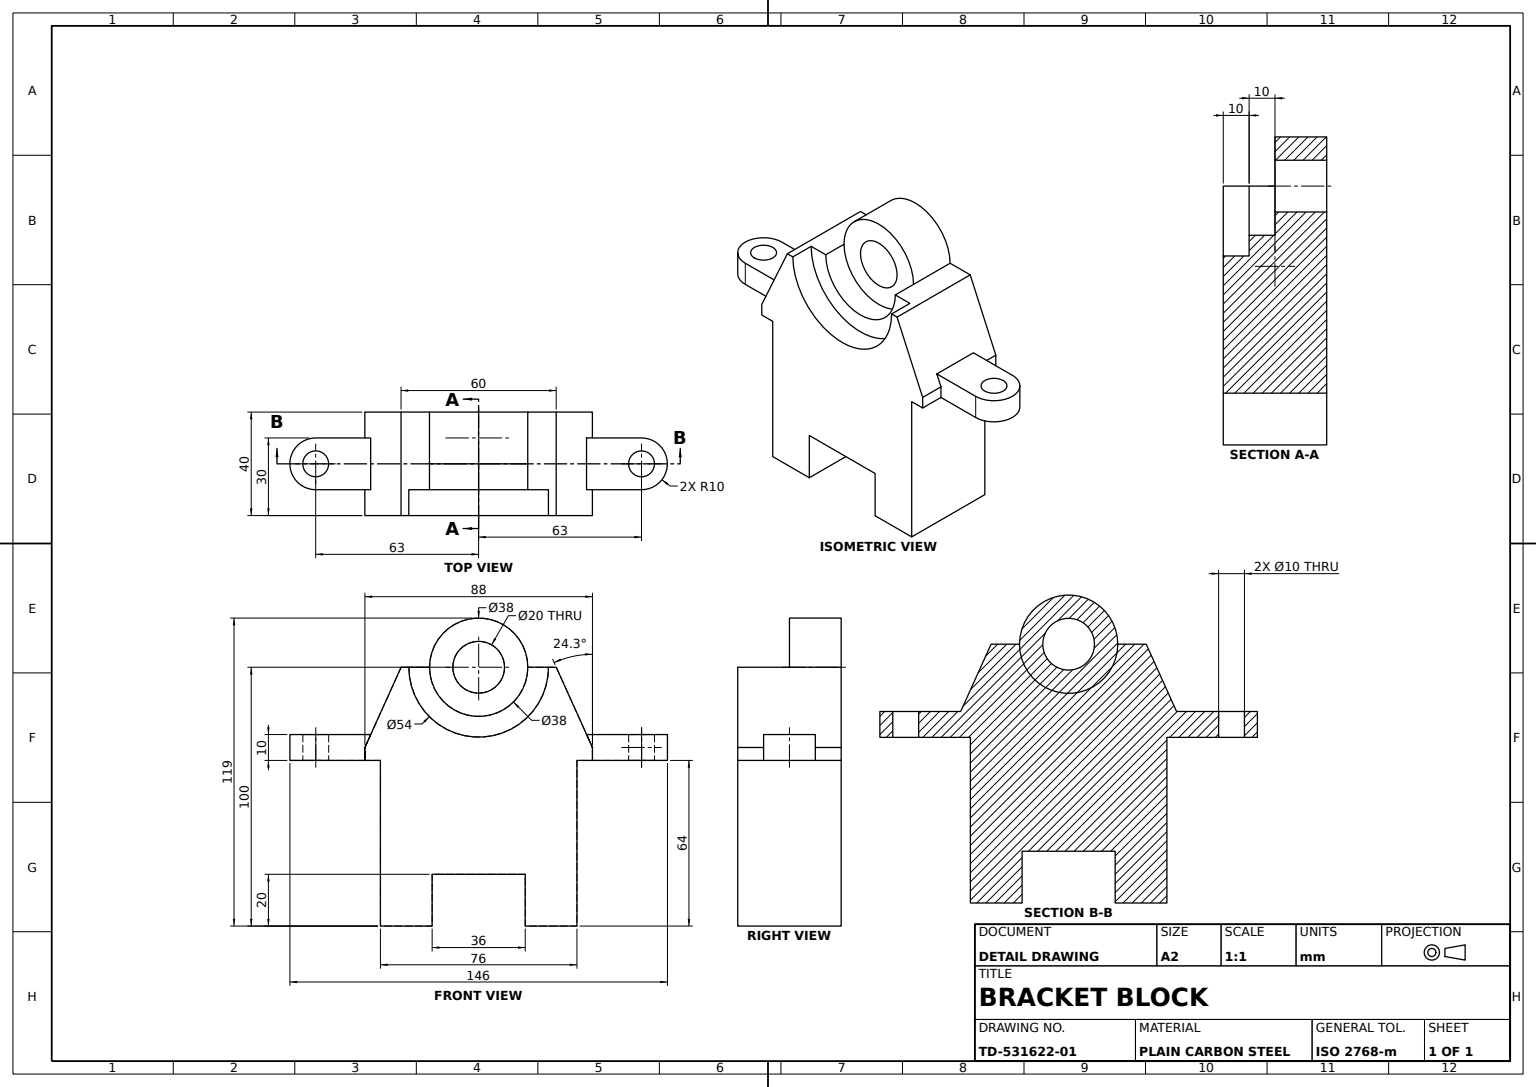
from build123d import *

# Parameters (mm, degrees)
PEDESTAL_BODY_DEPTH      = 20
FRONT_RECESS_54_SKETCH_R = 27
FRONT_RECESS_54_DEPTH    = 10
INNER_RECESS_38_SKETCH_R = 19
INNER_RECESS_38_DEPTH    = 10
HUB_38_SKETCH_R          = 19
HUB_38_DEPTH             = 20
BORE_20_SKETCH_R         = 10
BORE_20_DEPTH            = 100.523866484
MOUNTING_EAR_SKETCH_R    = 5
MOUNTING_EAR_DEPTH       = 10


with BuildPart() as part:
    # Pedestal Profile Sketch → Pedestal Body (new, symmetric)
    with BuildSketch(Plane.XY):
        Polygon((18, -32), (38, -32), (38, 32), (44, 32), (44, 37), (30, 68), (-30, 68), (-44, 37), (-44, 32), (-38, 32), (-38, -32), (-18, -32), (-18, -12), (18, -12), align=None)
    extrude(amount=PEDESTAL_BODY_DEPTH, both=True)

    # Front Recess Ø54 Sketch → Front Recess Ø54 (cut)
    with BuildSketch(Plane.XY.offset(20)):
        with Locations((0, 68)):
            Circle(FRONT_RECESS_54_SKETCH_R)
    extrude(amount=-FRONT_RECESS_54_DEPTH, mode=Mode.SUBTRACT)

    # Inner Recess Ø38 Sketch → Inner Recess Ø38 (cut)
    with BuildSketch(Plane.XY.offset(10)):
        with Locations((0, 68)):
            Circle(INNER_RECESS_38_SKETCH_R)
    extrude(amount=-INNER_RECESS_38_DEPTH, mode=Mode.SUBTRACT)

    # Hub Ø38 Sketch → Hub Ø38 (add)
    with BuildSketch(Plane.XY):
        with Locations((0, 68)):
            Circle(HUB_38_SKETCH_R)
    extrude(amount=-HUB_38_DEPTH)

    # Bore Ø20 Sketch → Bore Ø20 (cut, through all)
    with BuildSketch(Plane.XY):
        with Locations((0, 68)):
            Circle(BORE_20_SKETCH_R)
    extrude(amount=-BORE_20_DEPTH, mode=Mode.SUBTRACT)

    # Mounting Ear Sketch → Mounting Ear (add)
    with BuildSketch(Plane.XZ.offset(-32)):
        with BuildLine():
            Line((-63, 10), (-44, 10))
            Line((-44, 10), (-38, 10))
            Line((-38, 10), (-38, -10))
            Line((-38, -10), (-44, -10))
            Line((-44, -10), (-63, -10))
            ThreePointArc((-63, -10), (-73, 0), (-63, 10))
        make_face()
        with Locations(Location((-63, 0, 0), (0, 0, 270))):
            Circle(MOUNTING_EAR_SKETCH_R, mode=Mode.SUBTRACT)
    mounting_ear = extrude(amount=-MOUNTING_EAR_DEPTH)

    # Mounting Ear Mirror: Mounting Ear across plane
    add(mounting_ear.mirror(Plane(origin=(0, 0, 0), x_dir=(0, 0, 1), z_dir=(1, 0, 0))))


solid = part.part
